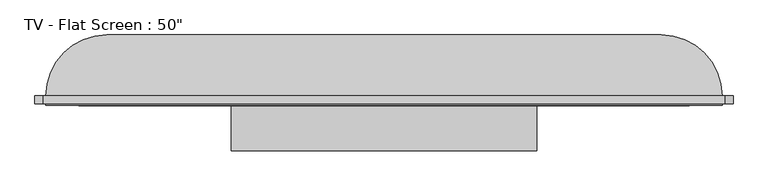
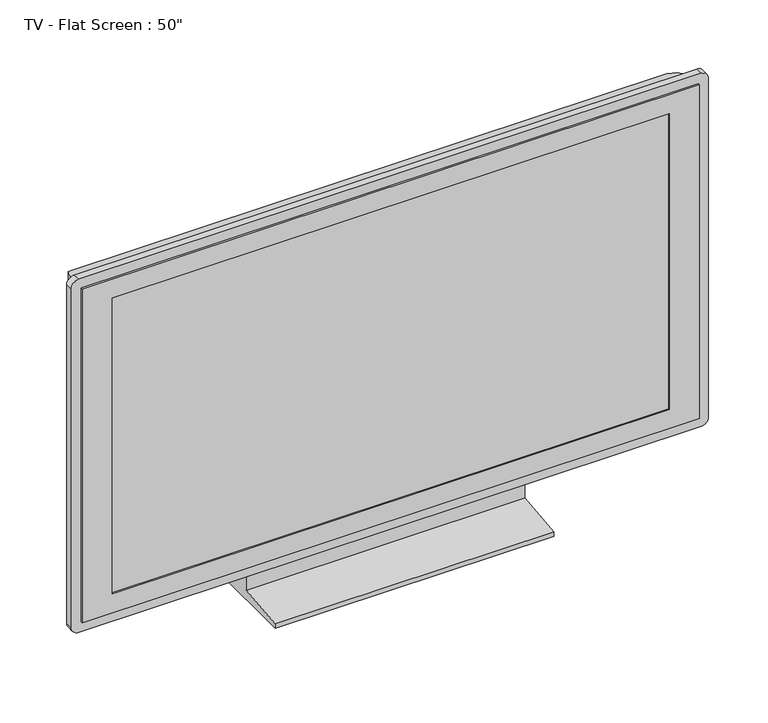
"""IFC4 building model written with IfcOpenShell, lengths in millimetres: furniture geometry."""

from ifc_helpers import new_model, si_unit, point, frame, frame_2d, origin, place, context, project, spatial, polyline, circle_curve, ellipse_curve, trimmed, segment, composite_curve, outline, extrude, faceted_brep, source, transform, mapped, element, save
from ifc_brep_helpers import plane_surface, cylinder_surface, advanced_brep


def furniture_fdf74506(model_context):
    return source(origin(), model_context, "Body", "SolidModel", [
        extrude(outline(polyline([(-51.4613764, 80.0), (-1.4613764, 80.0), (48.5386236, 0.0), (-151.4613764, 0.0), (-151.4613764, 10.0), (-51.4613764, 20.0), (-51.4613764, 80.0)])), frame((-280.6636439, 0.0, 0.0), z_axis=(1.0, 0.0, 0.0), x_axis=(0.0, 1.0, 0.0)), (0.0, 0.0, 1.0), 553.4382596),
        faceted_brep([(609.4937454, -69.4613764, 782.6751733), (-617.3827737, -69.4613764, 782.6751733), (-617.3827737, -69.4613764, 80.0), (609.4937454, -69.4613764, 80.0), (-557.3827737, -69.4613764, 742.6751733), (549.4937454, -69.4613764, 742.6751733), (549.4937454, -69.4613764, 120.0), (-557.3827737, -69.4613764, 120.0), (609.4937454, -51.4613764, 782.6751733), (609.4937454, -51.4613764, 80.0), (-617.3827737, -51.4613764, 80.0), (-617.3827737, -51.4613764, 782.6751733), (-557.3827737, -66.4613764, 742.6751733), (-557.3827737, -66.4613764, 120.0), (549.4937454, -66.4613764, 120.0), (549.4937454, -66.4613764, 742.6751733)], [[[0, 1, 2, 3], [4, 5, 6, 7]], [[8, 9, 10, 11]], [[1, 0, 8, 11]], [[2, 1, 11, 10]], [[3, 2, 10, 9]], [[0, 3, 9, 8]], [[12, 13, 14, 15]], [[12, 15, 5, 4]], [[15, 14, 6, 5]], [[14, 13, 7, 6]], [[13, 12, 4, 7]]]),
        extrude(outline(composite_curve([segment(polyline([(802.6751733, 614.4937454), (802.6751733, -622.3827737)]), True, "CONTINUOUS"), segment(trimmed(circle_curve(frame_2d((787.6751733, -622.3827737)), 15.0), [point((802.6751733, -622.3827737))], [point((787.6751733, -637.3827737))], False, "CARTESIAN"), True, "CONTINUOUS"), segment(polyline([(787.6751733, -637.3827737), (75.0, -637.3827737)]), True, "CONTINUOUS"), segment(trimmed(circle_curve(frame_2d((75.0, -622.3827737)), 15.0), [point((75.0, -637.3827737))], [point((60.0, -622.3827737))], False, "CARTESIAN"), True, "CONTINUOUS"), segment(polyline([(60.0, -622.3827737), (60.0, 614.4937454)]), True, "CONTINUOUS"), segment(trimmed(circle_curve(frame_2d((75.0, 614.4937454)), 15.0), [point((60.0, 614.4937454))], [point((75.0, 629.4937454))], False, "CARTESIAN"), True, "CONTINUOUS"), segment(polyline([(75.0, 629.4937454), (787.6751733, 629.4937454)]), True, "CONTINUOUS"), segment(trimmed(circle_curve(frame_2d((787.6751733, 614.4937454)), 15.0), [point((787.6751733, 629.4937454))], [point((802.6751733, 614.4937454))], False, "CARTESIAN"), True, "CONTINUOUS")], self_intersect=False), holes=[polyline([(782.6751733, 609.4937454), (80.0, 609.4937454), (80.0, -617.3827737), (782.6751733, -617.3827737), (782.6751733, 609.4937454)])]), frame((0.0, -66.4613764, 0.0), z_axis=(0.0, 1.0, 0.0), x_axis=(0.0, 0.0, 1.0)), (0.0, 0.0, 1.0), 15.0),
        advanced_brep(
        [(-617.3827737, -51.4613764, 80.0), (609.4937454, -51.4613764, 80.0), (609.4937454, -51.4613764, 782.6751733), (-617.3827737, -51.4613764, 782.6751733), (499.4937454, 58.5386236, 80.0), (-507.3827737, 58.5386236, 80.0), (-507.3827737, 58.5386236, 672.6751733), (499.4937454, 58.5386236, 672.6751733)],
        [
            (0, 1),
            (1, 2),
            (2, 3),
            (3, 0),
            (4, 5),
            (5, 6),
            (6, 7),
            (7, 4),
            (0, 5, circle_curve(frame((-507.3827737, -51.4613764, 80.0), z_axis=(0.0, 0.0, -1.0), x_axis=(-1.0, 0.0, 0.0)), 110.0)),
            (4, 1, circle_curve(frame((499.4937454, -51.4613764, 80.0), z_axis=(0.0, 0.0, -1.0), x_axis=(1.0, 0.0, 0.0)), 110.0)),
            (7, 2, ellipse_curve(frame((499.4937454, -51.4613764, 672.6751733), z_axis=(0.7071067811865475, 0.0, -0.7071067811865475), x_axis=(0.7071067811865474, 0.0, 0.7071067811865476)), 155.5634919, 110.0)),
            (6, 3, ellipse_curve(frame((-507.3827737, -51.4613764, 672.6751733), z_axis=(0.7071067811865475, 0.0, 0.7071067811865475), x_axis=(-0.7071067811865476, 0.0, 0.7071067811865474)), 155.5634919, 110.0)),
        ],
        [
            plane_surface(frame((-617.3827737, -51.4613764, 782.6751733), z_axis=(0.0, -1.0, 0.0), x_axis=(-1.0, 0.0, 0.0))),
            plane_surface(frame((-617.3827737, 58.5386236, 782.6751733), z_axis=(0.0, 1.0, 0.0), x_axis=(1.0, 0.0, 0.0))),
            plane_surface(frame((-617.3827737, -51.4613764, 80.0), z_axis=(0.0, 0.0, -1.0), x_axis=(0.0, 1.0, 0.0))),
            cylinder_surface(frame((499.4937454, -51.4613764, 80.0), z_axis=(0.0, 0.0, 1.0), x_axis=(1.0, 0.0, 0.0)), 110.0),
            cylinder_surface(frame((609.4937454, -51.4613764, 672.6751733), z_axis=(-1.0, 0.0, 0.0), x_axis=(0.0, 0.0, 1.0)), 110.0),
            cylinder_surface(frame((-507.3827737, -51.4613764, 782.6751733), z_axis=(0.0, 0.0, -1.0), x_axis=(-1.0, 0.0, 0.0)), 110.0),
        ],
        [
            (0, [[1, 2, 3, 4]]),
            (1, [[5, 6, 7, 8]]),
            (2, [[-1, 9, -5, 10]]),
            (3, [[11, -2, -10, -8]]),
            (4, [[-11, -7, 12, -3]]),
            (5, [[-12, -6, -9, -4]]),
        ],
    ),
    ])


if __name__ == "__main__":
    model = new_model("IFC4")
    model_context = context("Model", 3, world=origin())
    ifc_project = project(units=[si_unit("LENGTHUNIT", "METRE", prefix="MILLI")], contexts=[model_context])
    site = spatial("IfcSite", under=ifc_project)
    building = spatial("IfcBuilding", under=site)
    placement = place(None, origin())
    furniture_shape = furniture_fdf74506(model_context)
    element("IfcFurniture", 1, ObjectType="TV - Flat Screen : 50\"", at=placement, inside=building, context=model_context, shape_type="MappedRepresentation", body=[
        mapped(furniture_shape, transform((0.0, 0.0, 0.0), x_axis=(1.0, 0.0, 0.0), y_axis=(0.0, 1.0, 0.0), z_axis=(0.0, 0.0, 1.0))),
    ])
    save(model, "model.ifc")

# Revit data of these elements
# Type "TV - Flat Screen : 50\""
#   SinAng = 0' - 0.0193"
#   L = 3' - 7.57782"
#   H = 2' - 0.51477"
#   Thickness = 0' - 4.33071"
#   Diagonal = 4' - 2"
#   CosAng = 0' - 0.03431"
#   Stand [instance default] = yes
#   Default Elevation = 0
# Element 1 (IfcFurniture, "TV - Flat Screen : 50\"")
#   Materials on its faces: "TV - Black", "TV - Glass", "TV - Screen"
# Materials
#   "TV - Black": colour RGB 49 49 49, transparency 0
#   "TV - Glass": colour RGB 157 157 157, transparency 0.9
#   "TV - Screen": colour RGB 0 0 0, transparency 0
